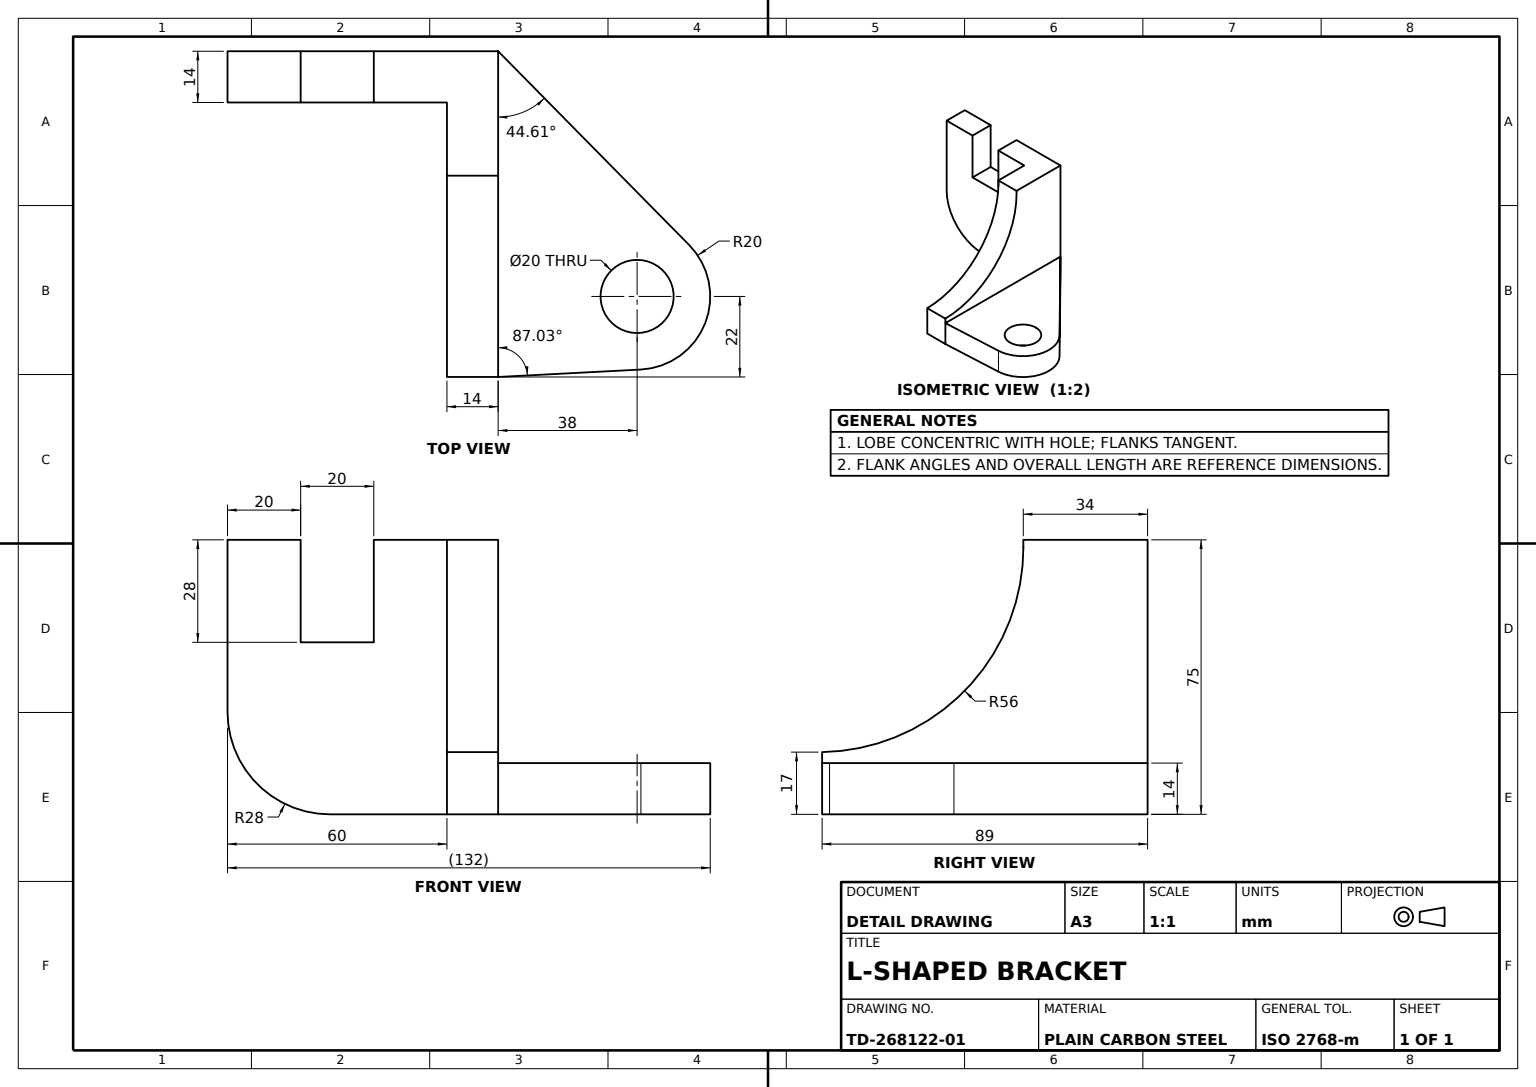
from build123d import *

# Parameters (mm, degrees)
BASE_PLATE_14MM_DEPTH        = 7
SIDE_PLATE_14MM_DEPTH        = 14
SLOTTED_END_PLATE_PROFILE_R  = 10
SLOTTED_END_PLATE_14MM_DEPTH = 14


with BuildPart() as part:
    # Base Plate Profile → Base Plate 14mm (new, symmetric)
    with BuildSketch(Plane.XY):
        with BuildLine():
            Line((0, 0), (0, 75))
            Line((0, 75), (32, 75))
            ThreePointArc((32, 75), (51.798989873, 66.798989873), (60, 47))
            Line((60, 47), (60, 0))
            Line((60, 0), (40, 0))
            Line((40, 0), (40, 28))
            Line((40, 28), (20, 28))
            Line((20, 28), (20, 0))
            Line((20, 0), (0, 0))
        make_face()
    extrude(amount=BASE_PLATE_14MM_DEPTH, both=True)

    # Side Plate Profile → Side Plate 14mm (add)
    with BuildSketch(Plane.ZY):
        with BuildLine():
            Line((-7, 75), (82, 75))
            Line((82, 75), (82, 58))
            ThreePointArc((82, 58), (42.329041508, 40.541426156), (27, 0))
            Line((27, 0), (7, 0))
            Line((7, 0), (-7, 0))
            Line((-7, 0), (-7, 75))
        make_face()
    extrude(amount=SIDE_PLATE_14MM_DEPTH)

    # Slotted End Plate Profile → Slotted End Plate 14mm (add)
    with BuildSketch(Plane(origin=(0, 75, 0), x_dir=(1, 0, 0), z_dir=(0, 1, 0))):
        with BuildLine():
            Line((-53.037054902, -79.973094831), (-14, -82))
            Line((-14, -82), (-14, 7))
            Line((-14, 7), (-66.238116475, -45.954501104))
            ThreePointArc((-66.238116475, -45.954501104), (-70.645345128, -67.23540635), (-53.037054902, -79.973094831))
        make_face()
        with Locations(Location((-52, -60, 0), (0, 0, 270))):
            Circle(SLOTTED_END_PLATE_PROFILE_R, mode=Mode.SUBTRACT)
    extrude(amount=-SLOTTED_END_PLATE_14MM_DEPTH)


solid = part.part
